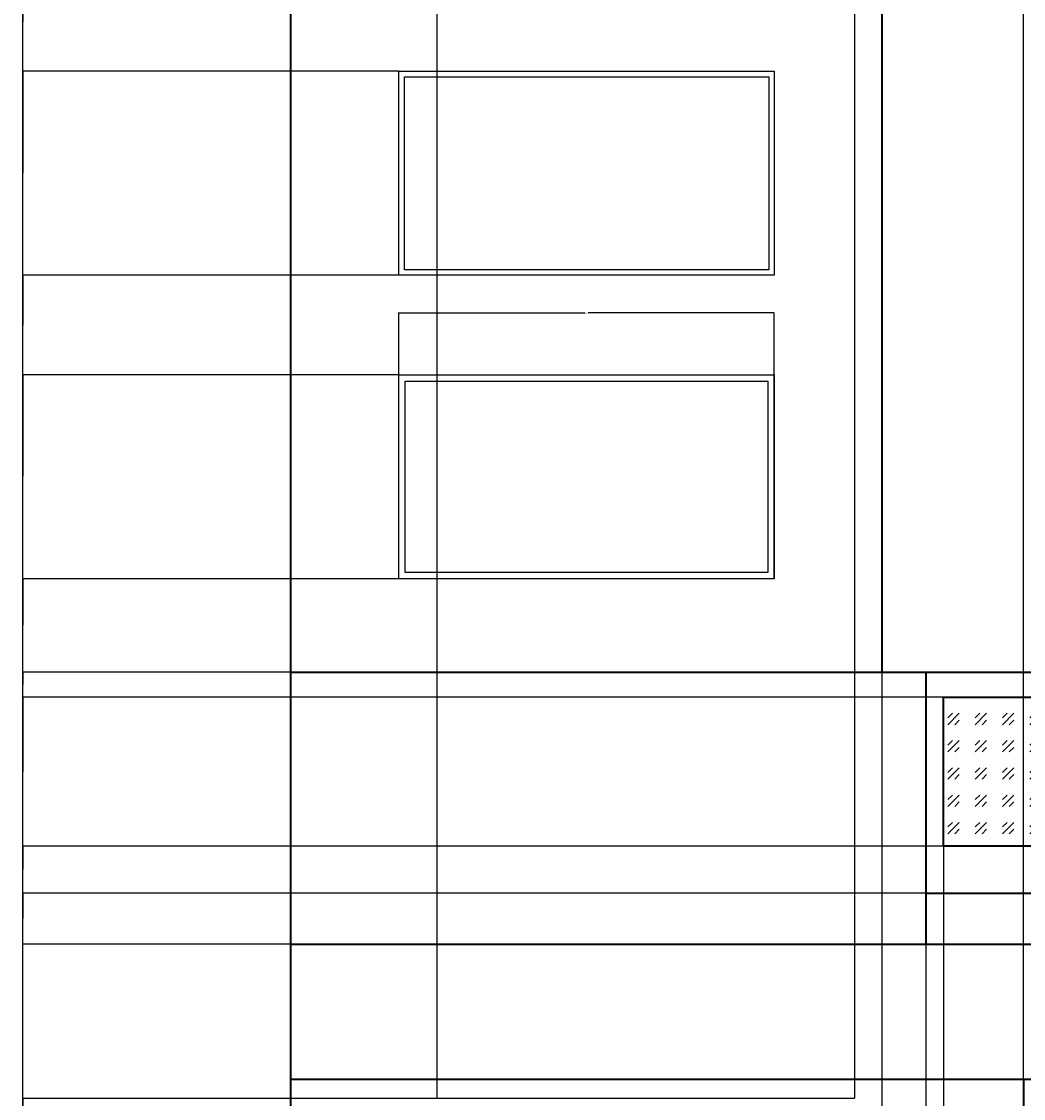
# Model space of a CAD drawing. Units: inches. Extents: x 1231 to 2151, y 481 to 2277.
# Tile 2 of 7: x 1231 to 1542, y 1038 to 1373. Entities that reach past the tile are written whole.
import ezdxf

# ---------------------------------------------------------------- set-up
doc = ezdxf.new("R2010")
doc.units = ezdxf.units.IN
doc.header["$MEASUREMENT"] = 0
for name, color, linetype, lineweight in [('A-ANNO-DIMS', 2, 'Continuous', 18), ('A-ELEV', 7, 'Continuous', 35), ('A-ELEV-PATT', 9, 'Continuous', 13), ('A-GLAZ', 3, 'Continuous', 25)]:
    doc.layers.add(name, color=color, linetype=linetype, lineweight=lineweight)
doc.styles.get("Standard").update_dxf_attribs({"font": 'arial.ttf'})
doc.dimstyles.get("Standard").update_dxf_attribs({"dimtxt": 0.18, "dimasz": 0.18, "dimexe": 0.18, "dimexo": 0.0625, "dimgap": 0.09, "dimtad": 0, "dimtih": 1, "dimtoh": 1, "dimdec": 0, "dimzin": 0, "dimdsep": 46, "dimlunit": 3, "dimtxsty": 'Standard', "dimcen": 0.09, "dimadec": 0, "dimazin": 0, "dimtfac": 1, "dimtdec": 0, "dimtofl": 0, "dimtmove": 0, "dimatfit": 3, "dimfxl": 1, "dimtolj": 1, "dimtzin": 0, "dimarcsym": 0})

# ---------------------------------------------------------------- blocks, each defined once
blk = doc.blocks.new('*D2')
at = {"layer": 'A-ANNO-DIMS', "color": 0, "lineweight": -2, "transparency": 16777216}
for p, q in [((1314.18, 2193.78), (1230.78, 2193.78)), ((1230.96, 2193.6), (1230.96, 1378.92)), ((1230.96, 563.87), (1230.96, 1378.55)), ((1314.18, 563.69), (1230.78, 563.69))]:
    blk.add_line(p, q, dxfattribs=at)
at = {"layer": 'A-ANNO-DIMS', "color": 0, "transparency": 16777216}
for points in [[(1230.93, 2193.6), (1230.99, 2193.6), (1230.96, 2193.78)], [(1230.93, 563.87), (1230.99, 563.87), (1230.96, 563.69)]]:
    blk.add_solid(points, dxfattribs=at)
at = {"layer": 'Defpoints', "color": 0, "transparency": 16777216}
for p in [(1230.96, 2193.78), (1314.24, 2193.78), (1314.24, 563.69)]:
    blk.add_point(p, dxfattribs=at)
at = {"layer": 'A-ANNO-DIMS', "color": 0, "transparency": 16777216, "insert": (1230.96, 1378.74), "char_height": 0.18, "attachment_point": 5}
blk.add_mtext('\\A1;1630', dxfattribs=at)
blk = doc.blocks.new('*D32')
at = {"layer": 'A-ANNO-DIMS', "color": 0, "lineweight": -2, "transparency": 16777216}
for p, q in [((1314.24, 1043.75), (1314.24, 2276.71)), ((1314.42, 2276.53), (1336.68, 2276.53)), ((1359.73, 2276.53), (1337.47, 2276.53)), ((1359.91, 1037.75), (1359.91, 2276.71))]:
    blk.add_line(p, q, dxfattribs=at)
at = {"layer": 'A-ANNO-DIMS', "color": 0, "transparency": 16777216}
for points in [[(1314.42, 2276.56), (1314.42, 2276.5), (1314.24, 2276.53)], [(1359.73, 2276.56), (1359.73, 2276.5), (1359.91, 2276.53)]]:
    blk.add_solid(points, dxfattribs=at)
at = {"layer": 'Defpoints', "color": 0, "transparency": 16777216}
for p in [(1359.91, 2276.53), (1314.24, 1043.69), (1359.91, 1037.69)]:
    blk.add_point(p, dxfattribs=at)
at = {"layer": 'A-ANNO-DIMS', "color": 0, "transparency": 16777216, "insert": (1337.07, 2276.53), "char_height": 0.18, "attachment_point": 5}
blk.add_mtext('\\A1;45.67', dxfattribs=at)
blk = doc.blocks.new('*D33')
at = {"layer": 'A-ANNO-DIMS', "color": 0, "lineweight": -2, "transparency": 16777216}
for p, q in [((1359.91, 1037.75), (1359.91, 2276.71)), ((1360.09, 2276.53), (1424.43, 2276.53)), ((1489.68, 2276.53), (1425.34, 2276.53)), ((1489.86, 1037.75), (1489.86, 2276.71))]:
    blk.add_line(p, q, dxfattribs=at)
at = {"layer": 'A-ANNO-DIMS', "color": 0, "transparency": 16777216}
for points in [[(1360.09, 2276.56), (1360.09, 2276.5), (1359.91, 2276.53)], [(1489.68, 2276.56), (1489.68, 2276.5), (1489.86, 2276.53)]]:
    blk.add_solid(points, dxfattribs=at)
at = {"layer": 'Defpoints', "color": 0, "transparency": 16777216}
for p in [(1489.86, 2276.53), (1359.91, 1037.69), (1489.86, 1037.69)]:
    blk.add_point(p, dxfattribs=at)
at = {"layer": 'A-ANNO-DIMS', "color": 0, "transparency": 16777216, "insert": (1424.88, 2276.53), "char_height": 0.18, "attachment_point": 5}
blk.add_mtext('\\A1;129.95', dxfattribs=at)
blk = doc.blocks.new('*D34')
at = {"layer": 'A-ANNO-DIMS', "color": 0, "lineweight": -2, "transparency": 16777216}
for p, q in [((1489.86, 1037.75), (1489.86, 2276.71)), ((1490.04, 2276.53), (1515.72, 2276.53)), ((1542.2, 2276.53), (1516.51, 2276.53)), ((1542.38, 1043.75), (1542.38, 2276.71))]:
    blk.add_line(p, q, dxfattribs=at)
at = {"layer": 'A-ANNO-DIMS', "color": 0, "transparency": 16777216}
for points in [[(1490.04, 2276.56), (1490.04, 2276.5), (1489.86, 2276.53)], [(1542.2, 2276.56), (1542.2, 2276.5), (1542.38, 2276.53)]]:
    blk.add_solid(points, dxfattribs=at)
at = {"layer": 'Defpoints', "color": 0, "transparency": 16777216}
for p in [(1542.38, 2276.53), (1542.38, 1043.69), (1489.86, 1037.69)]:
    blk.add_point(p, dxfattribs=at)
at = {"layer": 'A-ANNO-DIMS', "color": 0, "transparency": 16777216, "insert": (1516.12, 2276.53), "char_height": 0.18, "attachment_point": 5}
blk.add_mtext('\\A1;52.52', dxfattribs=at)
blk = doc.blocks.new('*D38')
at = {"layer": 'A-ANNO-DIMS', "color": 0, "lineweight": -2, "transparency": 16777216}
for p, q in [((1489.79, 1037.69), (1230.78, 1037.69)), ((1230.96, 1037.51), (1230.96, 992.91)), ((1230.96, 947.94), (1230.96, 992.54)), ((1489.79, 947.76), (1230.78, 947.76))]:
    blk.add_line(p, q, dxfattribs=at)
at = {"layer": 'A-ANNO-DIMS', "color": 0, "transparency": 16777216}
for points in [[(1230.93, 1037.51), (1230.99, 1037.51), (1230.96, 1037.69)], [(1230.93, 947.94), (1230.99, 947.94), (1230.96, 947.76)]]:
    blk.add_solid(points, dxfattribs=at)
at = {"layer": 'Defpoints', "color": 0, "transparency": 16777216}
for p in [(1230.96, 1037.69), (1489.86, 1037.69), (1489.86, 947.76)]:
    blk.add_point(p, dxfattribs=at)
at = {"layer": 'A-ANNO-DIMS', "color": 0, "transparency": 16777216, "insert": (1230.96, 992.72), "char_height": 0.18, "attachment_point": 5}
blk.add_mtext('\\A1;89.93', dxfattribs=at)
blk = doc.blocks.new('*D57')
at = {"layer": 'A-ANNO-DIMS', "color": 0, "lineweight": -2, "transparency": 16777216}
for p, q in [((1348.03, 1199.44), (1348.03, 1282.31)), ((1348.21, 1282.13), (1405.97, 1282.13)), ((1464.64, 1282.13), (1406.88, 1282.13)), ((1464.82, 1199.44), (1464.82, 1282.31))]:
    blk.add_line(p, q, dxfattribs=at)
at = {"layer": 'A-ANNO-DIMS', "color": 0, "transparency": 16777216}
for points in [[(1348.21, 1282.16), (1348.21, 1282.1), (1348.03, 1282.13)], [(1464.64, 1282.16), (1464.64, 1282.1), (1464.82, 1282.13)]]:
    blk.add_solid(points, dxfattribs=at)
at = {"layer": 'Defpoints', "color": 0, "transparency": 16777216}
for p in [(1464.82, 1282.13), (1348.03, 1199.38), (1464.82, 1199.38)]:
    blk.add_point(p, dxfattribs=at)
at = {"layer": 'A-ANNO-DIMS', "color": 0, "transparency": 16777216, "insert": (1406.42, 1282.13), "char_height": 0.18, "attachment_point": 5}
blk.add_mtext('\\A1;116.79', dxfattribs=at)
blk = doc.blocks.new('*D61')
at = {"layer": 'A-ANNO-DIMS', "color": 0, "lineweight": -2, "transparency": 16777216}
for p, q in [((1347.97, 1388.28), (1230.78, 1388.28)), ((1230.96, 1388.1), (1230.96, 1372.98)), ((1230.96, 1357.51), (1230.96, 1372.62)), ((1347.97, 1357.33), (1230.78, 1357.33))]:
    blk.add_line(p, q, dxfattribs=at)
at = {"layer": 'A-ANNO-DIMS', "color": 0, "transparency": 16777216}
for points in [[(1230.93, 1388.1), (1230.99, 1388.1), (1230.96, 1388.28)], [(1230.93, 1357.51), (1230.99, 1357.51), (1230.96, 1357.33)]]:
    blk.add_solid(points, dxfattribs=at)
at = {"layer": 'Defpoints', "color": 0, "transparency": 16777216}
for p in [(1348.03, 1388.28), (1230.96, 1357.33), (1348.03, 1357.33)]:
    blk.add_point(p, dxfattribs=at)
at = {"layer": 'A-ANNO-DIMS', "color": 0, "transparency": 16777216, "insert": (1230.96, 1372.8), "char_height": 0.18, "attachment_point": 5}
blk.add_mtext('\\A1;30.954', dxfattribs=at)
blk = doc.blocks.new('*D62')
at = {"layer": 'A-ANNO-DIMS', "color": 0, "lineweight": -2, "transparency": 16777216}
for p, q in [((1347.97, 1357.33), (1230.78, 1357.33)), ((1230.96, 1357.15), (1230.96, 1325.76)), ((1230.96, 1294.01), (1230.96, 1325.4)), ((1347.97, 1293.83), (1230.78, 1293.83))]:
    blk.add_line(p, q, dxfattribs=at)
at = {"layer": 'A-ANNO-DIMS', "color": 0, "transparency": 16777216}
for points in [[(1230.93, 1357.15), (1230.99, 1357.15), (1230.96, 1357.33)], [(1230.93, 1294.01), (1230.99, 1294.01), (1230.96, 1293.83)]]:
    blk.add_solid(points, dxfattribs=at)
at = {"layer": 'Defpoints', "color": 0, "transparency": 16777216}
for p in [(1348.03, 1357.33), (1230.96, 1293.83), (1348.03, 1293.83)]:
    blk.add_point(p, dxfattribs=at)
at = {"layer": 'A-ANNO-DIMS', "color": 0, "transparency": 16777216, "insert": (1230.96, 1325.58), "char_height": 0.18, "attachment_point": 5}
blk.add_mtext('\\A1;63.5', dxfattribs=at)
blk = doc.blocks.new('*D63')
at = {"layer": 'A-ANNO-DIMS', "color": 0, "lineweight": -2, "transparency": 16777216}
for p, q in [((1347.97, 1293.83), (1230.78, 1293.83)), ((1230.96, 1293.65), (1230.96, 1278.54)), ((1230.96, 1263.06), (1230.96, 1278.17)), ((1347.97, 1262.88), (1230.78, 1262.88))]:
    blk.add_line(p, q, dxfattribs=at)
at = {"layer": 'A-ANNO-DIMS', "color": 0, "transparency": 16777216}
for points in [[(1230.93, 1293.65), (1230.99, 1293.65), (1230.96, 1293.83)], [(1230.93, 1263.06), (1230.99, 1263.06), (1230.96, 1262.88)]]:
    blk.add_solid(points, dxfattribs=at)
at = {"layer": 'Defpoints', "color": 0, "transparency": 16777216}
for p in [(1348.03, 1293.83), (1230.96, 1262.88), (1348.03, 1262.88)]:
    blk.add_point(p, dxfattribs=at)
at = {"layer": 'A-ANNO-DIMS', "color": 0, "transparency": 16777216, "insert": (1230.96, 1278.35), "char_height": 0.18, "attachment_point": 5}
blk.add_mtext('\\A1;30.954', dxfattribs=at)
blk = doc.blocks.new('*D64')
at = {"layer": 'A-ANNO-DIMS', "color": 0, "lineweight": -2, "transparency": 16777216}
for p, q in [((1347.97, 1262.88), (1230.78, 1262.88)), ((1230.96, 1262.7), (1230.96, 1231.31)), ((1230.96, 1199.56), (1230.96, 1230.95)), ((1347.97, 1199.38), (1230.78, 1199.38))]:
    blk.add_line(p, q, dxfattribs=at)
at = {"layer": 'A-ANNO-DIMS', "color": 0, "transparency": 16777216}
for points in [[(1230.93, 1262.7), (1230.99, 1262.7), (1230.96, 1262.88)], [(1230.93, 1199.56), (1230.99, 1199.56), (1230.96, 1199.38)]]:
    blk.add_solid(points, dxfattribs=at)
at = {"layer": 'Defpoints', "color": 0, "transparency": 16777216}
for p in [(1348.03, 1262.88), (1230.96, 1199.38), (1348.03, 1199.38)]:
    blk.add_point(p, dxfattribs=at)
at = {"layer": 'A-ANNO-DIMS', "color": 0, "transparency": 16777216, "insert": (1230.96, 1231.13), "char_height": 0.18, "attachment_point": 5}
blk.add_mtext('\\A1;63.5', dxfattribs=at)
blk = doc.blocks.new('*D65')
at = {"layer": 'A-ANNO-DIMS', "color": 0, "lineweight": -2, "transparency": 16777216}
for p, q in [((1347.97, 1199.38), (1230.78, 1199.38)), ((1230.96, 1199.2), (1230.96, 1185.04)), ((1230.96, 1170.52), (1230.96, 1184.68)), ((1314.18, 1170.34), (1230.78, 1170.34))]:
    blk.add_line(p, q, dxfattribs=at)
at = {"layer": 'A-ANNO-DIMS', "color": 0, "transparency": 16777216}
for points in [[(1230.93, 1199.2), (1230.99, 1199.2), (1230.96, 1199.38)], [(1230.93, 1170.52), (1230.99, 1170.52), (1230.96, 1170.34)]]:
    blk.add_solid(points, dxfattribs=at)
at = {"layer": 'Defpoints', "color": 0, "transparency": 16777216}
for p in [(1348.03, 1199.38), (1230.96, 1170.34), (1314.24, 1170.34)]:
    blk.add_point(p, dxfattribs=at)
at = {"layer": 'A-ANNO-DIMS', "color": 0, "transparency": 16777216, "insert": (1230.96, 1184.86), "char_height": 0.18, "attachment_point": 5}
blk.add_mtext('\\A1;29.046', dxfattribs=at)
blk = doc.blocks.new('*D66')
at = {"layer": 'A-ANNO-DIMS', "color": 0, "lineweight": -2, "transparency": 16777216}
for p, q in [((1314.24, 1170.27), (1314.24, 480.76)), ((1498.31, 1170.27), (1498.31, 480.76)), ((1314.42, 480.94), (1405.82, 480.94)), ((1498.13, 480.94), (1406.73, 480.94))]:
    blk.add_line(p, q, dxfattribs=at)
at = {"layer": 'A-ANNO-DIMS', "color": 0, "transparency": 16777216}
for points in [[(1314.42, 480.97), (1314.42, 480.91), (1314.24, 480.94)], [(1498.13, 480.97), (1498.13, 480.91), (1498.31, 480.94)]]:
    blk.add_solid(points, dxfattribs=at)
at = {"layer": 'Defpoints', "color": 0, "transparency": 16777216}
for p in [(1314.24, 1170.34), (1498.31, 1170.34), (1498.31, 480.94)]:
    blk.add_point(p, dxfattribs=at)
at = {"layer": 'A-ANNO-DIMS', "color": 0, "transparency": 16777216, "insert": (1406.28, 480.94), "char_height": 0.18, "attachment_point": 5}
blk.add_mtext('\\A1;184.07', dxfattribs=at)
blk = doc.blocks.new('*D68')
at = {"layer": 'A-ANNO-DIMS', "color": 0, "lineweight": -2, "transparency": 16777216}
for p, q in [((1314.24, 1085.65), (1314.24, 480.76)), ((1512.01, 1085.65), (1512.01, 480.76)), ((1314.42, 480.94), (1412.67, 480.94)), ((1511.83, 480.94), (1413.58, 480.94))]:
    blk.add_line(p, q, dxfattribs=at)
at = {"layer": 'A-ANNO-DIMS', "color": 0, "transparency": 16777216}
for points in [[(1314.42, 480.97), (1314.42, 480.91), (1314.24, 480.94)], [(1511.83, 480.97), (1511.83, 480.91), (1512.01, 480.94)]]:
    blk.add_solid(points, dxfattribs=at)
at = {"layer": 'Defpoints', "color": 0, "transparency": 16777216}
for p in [(1314.24, 1085.71), (1512.01, 1085.71), (1512.01, 480.94)]:
    blk.add_point(p, dxfattribs=at)
at = {"layer": 'A-ANNO-DIMS', "color": 0, "transparency": 16777216, "insert": (1413.13, 480.94), "char_height": 0.18, "attachment_point": 5}
blk.add_mtext('\\A1;197.77', dxfattribs=at)
blk = doc.blocks.new('*D69')
at = {"layer": 'A-ANNO-DIMS', "color": 0, "lineweight": -2, "transparency": 16777216}
for p, q in [((1512.01, 1085.65), (1512.01, 480.76)), ((1937.57, 1085.65), (1937.57, 480.76)), ((1512.19, 480.94), (1724.39, 480.94)), ((1937.39, 480.94), (1725.19, 480.94))]:
    blk.add_line(p, q, dxfattribs=at)
at = {"layer": 'A-ANNO-DIMS', "color": 0, "transparency": 16777216}
for points in [[(1512.19, 480.97), (1512.19, 480.91), (1512.01, 480.94)], [(1937.39, 480.97), (1937.39, 480.91), (1937.57, 480.94)]]:
    blk.add_solid(points, dxfattribs=at)
at = {"layer": 'Defpoints', "color": 0, "transparency": 16777216}
for p in [(1512.01, 1085.71), (1937.57, 1085.71), (1937.57, 480.94)]:
    blk.add_point(p, dxfattribs=at)
at = {"layer": 'A-ANNO-DIMS', "color": 0, "transparency": 16777216, "insert": (1724.79, 480.94), "char_height": 0.18, "attachment_point": 5}
blk.add_mtext('\\A1;425.6', dxfattribs=at)
blk = doc.blocks.new('*D70')
at = {"layer": 'A-ANNO-DIMS', "color": 0, "lineweight": -2, "transparency": 16777216}
for p, q in [((1517.5, 1116.1), (1517.5, 480.76)), ((1512.01, 1101.52), (1512.01, 480.76)), ((1512.19, 480.94), (1514.36, 480.94)), ((1517.32, 480.94), (1515.15, 480.94))]:
    blk.add_line(p, q, dxfattribs=at)
at = {"layer": 'A-ANNO-DIMS', "color": 0, "transparency": 16777216}
for points in [[(1512.19, 480.97), (1512.19, 480.91), (1512.01, 480.94)], [(1517.32, 480.97), (1517.32, 480.91), (1517.5, 480.94)]]:
    blk.add_solid(points, dxfattribs=at)
at = {"layer": 'Defpoints', "color": 0, "transparency": 16777216}
for p in [(1517.5, 1116.16), (1512.01, 1101.58), (1517.5, 480.94)]:
    blk.add_point(p, dxfattribs=at)
at = {"layer": 'A-ANNO-DIMS', "color": 0, "transparency": 16777216, "insert": (1514.76, 480.94), "char_height": 0.18, "attachment_point": 5}
blk.add_mtext('\\A1;5.493', dxfattribs=at)
blk = doc.blocks.new('*D71')
at = {"layer": 'A-ANNO-DIMS', "color": 0, "lineweight": -2, "transparency": 16777216}
for p, q in [((1517.5, 1116.1), (1517.5, 480.76)), ((1595.89, 1116.1), (1595.89, 480.76)), ((1517.68, 480.94), (1556.31, 480.94)), ((1595.71, 480.94), (1557.09, 480.94))]:
    blk.add_line(p, q, dxfattribs=at)
at = {"layer": 'A-ANNO-DIMS', "color": 0, "transparency": 16777216}
for points in [[(1517.68, 480.97), (1517.68, 480.91), (1517.5, 480.94)], [(1595.71, 480.97), (1595.71, 480.91), (1595.89, 480.94)]]:
    blk.add_solid(points, dxfattribs=at)
at = {"layer": 'Defpoints', "color": 0, "transparency": 16777216}
for p in [(1517.5, 1116.16), (1595.89, 1116.16), (1595.89, 480.94)]:
    blk.add_point(p, dxfattribs=at)
at = {"layer": 'A-ANNO-DIMS', "color": 0, "transparency": 16777216, "insert": (1556.7, 480.94), "char_height": 0.18, "attachment_point": 5}
blk.add_mtext('\\A1;78.39', dxfattribs=at)
blk = doc.blocks.new('*D76')
at = {"layer": 'A-ANNO-DIMS', "color": 0, "lineweight": -2, "transparency": 16777216}
for p, q in [((1511.95, 1101.58), (1230.78, 1101.58)), ((1230.96, 1101.4), (1230.96, 1093.83)), ((1230.96, 1085.89), (1230.96, 1093.46)), ((1511.95, 1085.71), (1230.78, 1085.71))]:
    blk.add_line(p, q, dxfattribs=at)
at = {"layer": 'A-ANNO-DIMS', "color": 0, "transparency": 16777216}
for points in [[(1230.93, 1101.4), (1230.99, 1101.4), (1230.96, 1101.58)], [(1230.93, 1085.89), (1230.99, 1085.89), (1230.96, 1085.71)]]:
    blk.add_solid(points, dxfattribs=at)
at = {"layer": 'Defpoints', "color": 0, "transparency": 16777216}
for p in [(1230.96, 1101.58), (1512.01, 1101.58), (1512.01, 1085.71)]:
    blk.add_point(p, dxfattribs=at)
at = {"layer": 'A-ANNO-DIMS', "color": 0, "transparency": 16777216, "insert": (1230.96, 1093.65), "char_height": 0.18, "attachment_point": 5}
blk.add_mtext('\\A1;15.875', dxfattribs=at)
blk = doc.blocks.new('*D77')
at = {"layer": 'A-ANNO-DIMS', "color": 0, "lineweight": -2, "transparency": 16777216}
for p, q in [((1517.44, 1116.16), (1230.78, 1116.16)), ((1230.96, 1115.98), (1230.96, 1109.05)), ((1230.96, 1101.76), (1230.96, 1108.69)), ((1511.95, 1101.58), (1230.78, 1101.58))]:
    blk.add_line(p, q, dxfattribs=at)
at = {"layer": 'A-ANNO-DIMS', "color": 0, "transparency": 16777216}
for points in [[(1230.93, 1115.98), (1230.99, 1115.98), (1230.96, 1116.16)], [(1230.93, 1101.76), (1230.99, 1101.76), (1230.96, 1101.58)]]:
    blk.add_solid(points, dxfattribs=at)
at = {"layer": 'Defpoints', "color": 0, "transparency": 16777216}
for p in [(1230.96, 1116.16), (1517.5, 1116.16), (1512.01, 1101.58)]:
    blk.add_point(p, dxfattribs=at)
at = {"layer": 'A-ANNO-DIMS', "color": 0, "transparency": 16777216, "insert": (1230.96, 1108.87), "char_height": 0.18, "attachment_point": 5}
blk.add_mtext('\\A1;14.576', dxfattribs=at)
blk = doc.blocks.new('*D78')
at = {"layer": 'A-ANNO-DIMS', "color": 0, "lineweight": -2, "transparency": 16777216}
for p, q in [((1517.44, 1162.6), (1230.78, 1162.6)), ((1230.96, 1162.42), (1230.96, 1139.56)), ((1230.96, 1116.34), (1230.96, 1139.2)), ((1517.44, 1116.16), (1230.78, 1116.16))]:
    blk.add_line(p, q, dxfattribs=at)
at = {"layer": 'A-ANNO-DIMS', "color": 0, "transparency": 16777216}
for points in [[(1230.93, 1162.42), (1230.99, 1162.42), (1230.96, 1162.6)], [(1230.93, 1116.34), (1230.99, 1116.34), (1230.96, 1116.16)]]:
    blk.add_solid(points, dxfattribs=at)
at = {"layer": 'Defpoints', "color": 0, "transparency": 16777216}
for p in [(1230.96, 1162.6), (1517.5, 1162.6), (1517.5, 1116.16)]:
    blk.add_point(p, dxfattribs=at)
at = {"layer": 'A-ANNO-DIMS', "color": 0, "transparency": 16777216, "insert": (1230.96, 1139.38), "char_height": 0.18, "attachment_point": 5}
blk.add_mtext('\\A1;46.44', dxfattribs=at)
blk = doc.blocks.new('*D79')
at = {"layer": 'A-ANNO-DIMS', "color": 0, "lineweight": -2, "transparency": 16777216}
for p, q in [((1511.95, 1170.34), (1230.78, 1170.34)), ((1230.96, 1170.16), (1230.96, 1166.65)), ((1230.96, 1162.78), (1230.96, 1166.28)), ((1517.44, 1162.6), (1230.78, 1162.6))]:
    blk.add_line(p, q, dxfattribs=at)
at = {"layer": 'A-ANNO-DIMS', "color": 0, "transparency": 16777216}
for points in [[(1230.93, 1170.16), (1230.99, 1170.16), (1230.96, 1170.34)], [(1230.93, 1162.78), (1230.99, 1162.78), (1230.96, 1162.6)]]:
    blk.add_solid(points, dxfattribs=at)
at = {"layer": 'Defpoints', "color": 0, "transparency": 16777216}
for p in [(1230.96, 1170.34), (1512.01, 1170.34), (1517.5, 1162.6)]:
    blk.add_point(p, dxfattribs=at)
at = {"layer": 'A-ANNO-DIMS', "color": 0, "transparency": 16777216, "insert": (1230.96, 1166.47), "char_height": 0.18, "attachment_point": 5}
blk.add_mtext('\\A1;7.739', dxfattribs=at)

msp = doc.modelspace()

# ---------------------------------------------------------------- hatches: boundary and pattern name
at = {"layer": 'A-ELEV-PATT'}
h = msp.add_hatch(dxfattribs=at)
h.set_pattern_fill('GOST_GLASS', color=256)
h.set_pattern_definition([(45, (0, 0), (8.485281, 0), [5, -7]), (45, (2.1213, 0), (8.485281, 0), [2, -10]), (45, (0, 2.1213), (8.485281, 0), [2, -10])])
h.paths.add_polyline_path([(1595.8928, 1116.1584), (1595.8928, 1162.5965), (1517.5039, 1162.5965), (1517.5039, 1116.1584)])
h.paths.add_polyline_path([(1689.5303, 1162.5965), (1611.1414, 1162.5965), (1611.1414, 1116.1584), (1689.5303, 1116.1584)])
h.paths.add_polyline_path([(1933.3556, 1116.1584), (1933.3556, 1162.5965), (1701.522, 1162.5965), (1701.522, 1116.1584)])

# ---------------------------------------------------------------- linework, layer by layer
at = {"layer": 'A-ELEV'}
for p, q in [((1314.2408, 1926.2862), (1314.2408, 563.6912)), ((1498.3132, 1475.5441), (1498.3132, 1170.3351)), ((1314.2408, 1170.3351), (2067.6855, 1170.3351)), ((1512.0105, 1170.3351), (1512.0105, 1085.7079)), ((1512.0105, 1101.5825), (1937.5725, 1101.5825)), ((1314.2408, 1085.7079), (2067.6855, 1085.7079)), ((1314.2408, 1043.6912), (2067.6855, 1043.6912)), ((1542.3752, 1043.6912), (1542.3752, 563.6912))]:
    msp.add_line(p, q, dxfattribs=at)
msp.add_lwpolyline([(1517.5039, 1162.5965), (1595.8928, 1162.5965), (1595.8928, 1116.1584), (1517.5039, 1116.1584)], close=True, dxfattribs=at)
at = {"layer": 'A-GLAZ'}
for points in [[(1348.0309, 1357.3253), (1464.8184, 1357.3253), (1464.8184, 1293.8301), (1348.0309, 1293.8301)], [(1349.7283, 1355.6279), (1463.121, 1355.6279), (1463.121, 1295.5275), (1349.7283, 1295.5275)], [(1348.0309, 1262.8765), (1464.8184, 1262.8765), (1464.8184, 1199.3812), (1348.0309, 1199.3812)], [(1349.9884, 1260.919), (1462.8609, 1260.919), (1462.8609, 1201.3387), (1349.9884, 1201.3387)]]:
    msp.add_lwpolyline(points, close=True, dxfattribs=at)

# ---------------------------------------------------------------- dimensions: what is measured, and where the dimension line sits
at = {"layer": 'A-ANNO-DIMS'}
for base, p1, p2, override, picture, middle in [((1359.9075, 2276.5289), (1314.2408, 1043.6912), (1359.9075, 1037.6872), {"dimdec": 2, "dimlfac": 1, "dimrnd": 0, "dimzin": 0, "dimdsep": 46, "dimlunit": 2}, '*D32', (1337.0741, 2276.5289)), ((1489.8565, 2276.5289), (1359.9075, 1037.6872), (1489.8565, 1037.6872), {"dimdec": 2, "dimlfac": 1, "dimrnd": 0, "dimzin": 0, "dimdsep": 46, "dimlunit": 2}, '*D33', (1424.882, 2276.5289)), ((1542.3752, 2276.5289), (1489.8565, 1037.6872), (1542.3752, 1043.6912), {"dimdec": 2, "dimlfac": 1, "dimrnd": 0, "dimzin": 0, "dimdsep": 46, "dimlunit": 2}, '*D34', (1516.1158, 2276.5289)), ((1464.8184, 1282.1312), (1348.0309, 1199.3812), (1464.8184, 1199.3812), {"dimdec": 2, "dimlfac": 1, "dimrnd": 0, "dimzin": 0, "dimdsep": 46, "dimlunit": 2}, '*D57', (1406.4246, 1282.1312)), ((1498.3132, 480.9412), (1314.2408, 1170.3351), (1498.3132, 1170.3351), {"dimdec": 2, "dimlfac": 1, "dimrnd": 0, "dimzin": 0, "dimdsep": 46, "dimlunit": 2}, '*D66', (1406.277, 480.9412)), ((1517.5039, 480.9412), (1512.0105, 1101.5825), (1517.5039, 1116.1584), {"dimdec": 3, "dimlfac": 1, "dimrnd": 0, "dimzin": 0, "dimdsep": 46, "dimlunit": 2}, '*D70', (1514.7572, 480.9412)), ((1595.8928, 480.9412), (1517.5039, 1116.1584), (1595.8928, 1116.1584), {"dimdec": 2, "dimlfac": 1, "dimrnd": 0, "dimzin": 0, "dimdsep": 46, "dimlunit": 2}, '*D71', (1556.6984, 480.9412)), ((1512.0105, 480.9412), (1314.2408, 1085.7079), (1512.0105, 1085.7079), {"dimdec": 2, "dimlfac": 1, "dimrnd": 0, "dimzin": 0, "dimdsep": 46, "dimlunit": 2}, '*D68', (1413.1257, 480.9412)), ((1937.5725, 480.9412), (1512.0105, 1085.7079), (1937.5725, 1085.7079), {"dimdec": 1, "dimlfac": 1, "dimrnd": 0, "dimzin": 0, "dimdsep": 46, "dimlunit": 2}, '*D69', (1724.7915, 480.9412))]:
    dim = msp.add_linear_dim(base=base, p1=p1, p2=p2, dimstyle='Standard', override=override, dxfattribs=at)
    dim.commit()
    dim.dimension.update_dxf_attribs({"geometry": picture, "text_midpoint": middle})
for base, p1, p2, override, picture, middle in [((1230.9629, 2193.7789), (1314.2408, 563.6912), (1314.2408, 2193.7789), {"dimdec": 0, "dimlfac": 1, "dimrnd": 0, "dimzin": 0, "dimdsep": 46, "dimlunit": 2}, '*D2', (1230.9629, 1378.7351)), ((1230.9629, 1357.3253), (1348.0309, 1388.2789), (1348.0309, 1357.3253), {"dimdec": 3, "dimlfac": 1, "dimrnd": 0, "dimzin": 0, "dimdsep": 46, "dimlunit": 2}, '*D61', (1230.9629, 1372.8021)), ((1230.9629, 1293.8301), (1348.0309, 1357.3253), (1348.0309, 1293.8301), {"dimdec": 1, "dimlfac": 1, "dimrnd": 0, "dimzin": 0, "dimdsep": 46, "dimlunit": 2}, '*D62', (1230.9629, 1325.5777)), ((1230.9629, 1262.8765), (1348.0309, 1293.8301), (1348.0309, 1262.8765), {"dimdec": 3, "dimlfac": 1, "dimrnd": 0, "dimzin": 0, "dimdsep": 46, "dimlunit": 2}, '*D63', (1230.9629, 1278.3533)), ((1230.9629, 1199.3812), (1348.0309, 1262.8765), (1348.0309, 1199.3812), {"dimdec": 1, "dimlfac": 1, "dimrnd": 0, "dimzin": 0, "dimdsep": 46, "dimlunit": 2}, '*D64', (1230.9629, 1231.1288)), ((1230.9629, 1170.3351), (1348.0309, 1199.3812), (1314.2408, 1170.3351), {"dimdec": 3, "dimlfac": 1, "dimrnd": 0, "dimzin": 0, "dimdsep": 46, "dimlunit": 2}, '*D65', (1230.9629, 1184.8582)), ((1230.9629, 1170.3351), (1517.5039, 1162.5965), (1512.0105, 1170.3351), {"dimdec": 3, "dimlfac": 1, "dimrnd": 0, "dimzin": 0, "dimdsep": 46, "dimlunit": 2}, '*D79', (1230.9629, 1166.4658)), ((1230.9629, 1162.5965), (1517.5039, 1116.1584), (1517.5039, 1162.5965), {"dimdec": 2, "dimlfac": 1, "dimrnd": 0, "dimzin": 0, "dimdsep": 46, "dimlunit": 2}, '*D78', (1230.9629, 1139.3774)), ((1230.9629, 1116.1584), (1512.0105, 1101.5825), (1517.5039, 1116.1584), {"dimdec": 3, "dimlfac": 1, "dimrnd": 0, "dimzin": 0, "dimdsep": 46, "dimlunit": 2}, '*D77', (1230.9629, 1108.8704)), ((1230.9629, 1101.5825), (1512.0105, 1085.7079), (1512.0105, 1101.5825), {"dimdec": 3, "dimlfac": 1, "dimrnd": 0, "dimzin": 0, "dimdsep": 46, "dimlunit": 2}, '*D76', (1230.9629, 1093.6452)), ((1230.9629, 1037.6872), (1489.8565, 947.7593), (1489.8565, 1037.6872), {"dimdec": 2, "dimlfac": 1, "dimrnd": 0, "dimzin": 0, "dimdsep": 46, "dimlunit": 2}, '*D38', (1230.9629, 992.7232))]:
    dim = msp.add_linear_dim(base=base, p1=p1, p2=p2, angle=90, dimstyle='Standard', override=override, dxfattribs=at)
    dim.commit()
    dim.dimension.update_dxf_attribs({"geometry": picture, "text_midpoint": middle})

doc.saveas('drawing.dxf')
